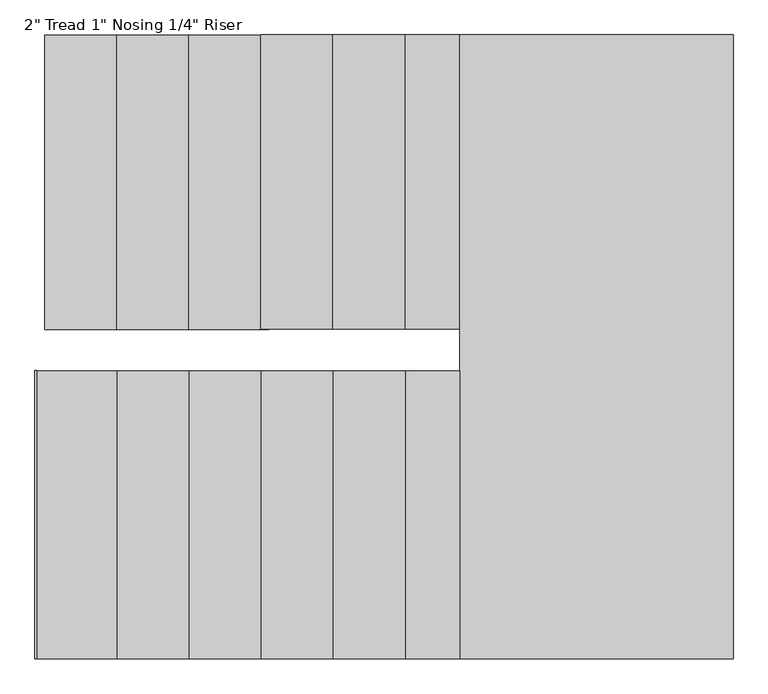
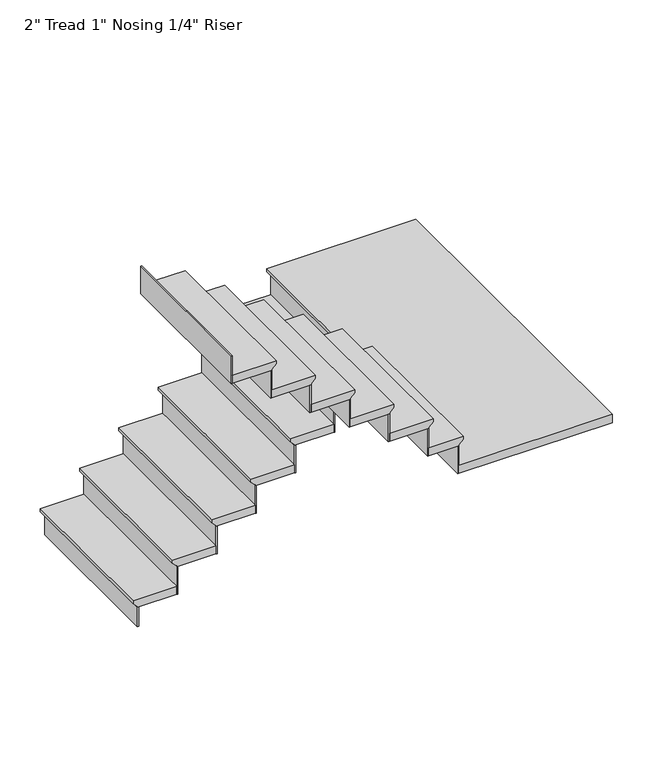
"""IFC4 building model written with IfcOpenShell, lengths in millimetres: stair flight geometry."""

from ifc_helpers import new_model, si_unit, origin, place, context, project, spatial, faceted_brep, source, transform, mapped, element, save


def stair_flight_3a0fea93(model_context):
    return source(origin(), model_context, "Body", "Brep", [
        faceted_brep([(-1022.6415352, -3861.2539367, 150.2833333), (-1022.6415352, -3861.2539367, 169.3333333), (-1022.6415352, -2926.4769687, 169.3333333), (-1022.6415352, -2926.4769687, 150.2833333), (-997.2415352, -3861.2539367, 124.8833333), (-997.2415352, -2926.4769687, 124.8833333), (-768.6415352, -3861.2539367, 169.3333333), (-768.6415352, -2926.4769687, 169.3333333), (-997.2415352, -2926.4769687, 118.5333333), (-768.6415352, -2926.4769687, 118.5333333), (-768.6415352, -3861.2539367, 118.5333333), (-997.2415352, -3861.2539367, 118.5333333)], [[[0, 1, 2, 3]], [[4, 0, 3, 5]], [[2, 1, 6, 7]], [[8, 9, 10, 11]], [[2, 7, 9, 8, 5, 3]], [[8, 11, 4, 5]], [[6, 1, 0, 4, 11, 10]], [[7, 6, 10, 9]]]),
        faceted_brep([(-997.2415352, -3861.2539367, 118.5333333), (-997.2415352, -3861.2539367, 0.0), (-990.8915352, -3861.2539367, 0.0), (-990.8915352, -3861.2539367, 118.5333333), (-997.2415352, -2926.4769687, 118.5333333), (-990.8915352, -2926.4769687, 118.5333333), (-990.8915352, -2926.4769687, 0.0), (-997.2415352, -2926.4769687, 0.0)], [[[0, 1, 2, 3]], [[4, 5, 6, 7]], [[1, 0, 4, 7]], [[2, 1, 7, 6]], [[3, 2, 6, 5]], [[0, 3, 5, 4]]]),
        faceted_brep([(-768.6415352, -3861.2539367, 287.8666667), (-768.6415352, -3861.2539367, 118.5333333), (-762.2915352, -3861.2539367, 118.5333333), (-762.2915352, -3861.2539367, 287.8666667), (-768.6415352, -2926.4769687, 287.8666667), (-762.2915352, -2926.4769687, 287.8666667), (-762.2915352, -2926.4769687, 118.5333333), (-768.6415352, -2926.4769687, 118.5333333)], [[[0, 1, 2, 3]], [[4, 5, 6, 7]], [[1, 0, 4, 7]], [[2, 1, 7, 6]], [[3, 2, 6, 5]], [[0, 3, 5, 4]]]),
        faceted_brep([(-794.0415352, -2926.4769687, 338.6666667), (-794.0415352, -3861.2539367, 338.6666667), (-540.0415352, -3861.2539367, 338.6666667), (-540.0415352, -2926.4769687, 338.6666667), (-768.6415352, -2926.4769687, 287.8666667), (-540.0415352, -2926.4769687, 287.8666667), (-540.0415352, -3861.2539367, 287.8666667), (-768.6415352, -3861.2539367, 287.8666667), (-768.6415352, -2926.4769687, 294.2166667), (-794.0415352, -2926.4769687, 319.6166667), (-768.6415352, -3861.2539367, 294.2166667), (-794.0415352, -3861.2539367, 319.6166667)], [[[0, 1, 2, 3]], [[4, 5, 6, 7]], [[0, 3, 5, 4, 8, 9]], [[4, 7, 10, 8]], [[2, 1, 11, 10, 7, 6]], [[3, 2, 6, 5]], [[11, 1, 0, 9]], [[10, 11, 9, 8]]]),
        faceted_brep([(-540.0415352, -3861.2539367, 457.2), (-540.0415352, -3861.2539367, 287.8666667), (-533.6915352, -3861.2539367, 287.8666667), (-533.6915352, -3861.2539367, 457.2), (-540.0415352, -2926.4769687, 457.2), (-533.6915352, -2926.4769687, 457.2), (-533.6915352, -2926.4769687, 287.8666667), (-540.0415352, -2926.4769687, 287.8666667)], [[[0, 1, 2, 3]], [[4, 5, 6, 7]], [[1, 0, 4, 7]], [[2, 1, 7, 6]], [[3, 2, 6, 5]], [[0, 3, 5, 4]]]),
        faceted_brep([(-565.4415352, -2926.4769687, 508.0), (-565.4415352, -3861.2539367, 508.0), (-311.4415352, -3861.2539367, 508.0), (-311.4415352, -2926.4769687, 508.0), (-540.0415352, -2926.4769687, 457.2), (-311.4415352, -2926.4769687, 457.2), (-311.4415352, -3861.2539367, 457.2), (-540.0415352, -3861.2539367, 457.2), (-540.0415352, -2926.4769687, 463.55), (-565.4415352, -2926.4769687, 488.95), (-540.0415352, -3861.2539367, 463.55), (-565.4415352, -3861.2539367, 488.95)], [[[0, 1, 2, 3]], [[4, 5, 6, 7]], [[0, 3, 5, 4, 8, 9]], [[4, 7, 10, 8]], [[2, 1, 11, 10, 7, 6]], [[3, 2, 6, 5]], [[11, 1, 0, 9]], [[10, 11, 9, 8]]]),
        faceted_brep([(-311.4415352, -3861.2539367, 626.5333333), (-311.4415352, -3861.2539367, 457.2), (-305.0915352, -3861.2539367, 457.2), (-305.0915352, -3861.2539367, 626.5333333), (-311.4415352, -2926.4769687, 626.5333333), (-305.0915352, -2926.4769687, 626.5333333), (-305.0915352, -2926.4769687, 457.2), (-311.4415352, -2926.4769687, 457.2)], [[[0, 1, 2, 3]], [[4, 5, 6, 7]], [[1, 0, 4, 7]], [[2, 1, 7, 6]], [[3, 2, 6, 5]], [[0, 3, 5, 4]]]),
        faceted_brep([(-336.8415352, -2926.4769687, 677.3333333), (-336.8415352, -3861.2539367, 677.3333333), (-82.8415352, -3861.2539367, 677.3333333), (-82.8415352, -2926.4769687, 677.3333333), (-311.4415352, -2926.4769687, 626.5333333), (-82.8415352, -2926.4769687, 626.5333333), (-82.8415352, -3861.2539367, 626.5333333), (-311.4415352, -3861.2539367, 626.5333333), (-311.4415352, -2926.4769687, 632.8833333), (-336.8415352, -2926.4769687, 658.2833333), (-311.4415352, -3861.2539367, 632.8833333), (-336.8415352, -3861.2539367, 658.2833333)], [[[0, 1, 2, 3]], [[4, 5, 6, 7]], [[0, 3, 5, 4, 8, 9]], [[4, 7, 10, 8]], [[2, 1, 11, 10, 7, 6]], [[3, 2, 6, 5]], [[11, 1, 0, 9]], [[10, 11, 9, 8]]]),
        faceted_brep([(-82.8415352, -3861.2539367, 795.8666667), (-82.8415352, -3861.2539367, 626.5333333), (-76.4915352, -3861.2539367, 626.5333333), (-76.4915352, -3861.2539367, 795.8666667), (-82.8415352, -2926.4769687, 795.8666667), (-76.4915352, -2926.4769687, 795.8666667), (-76.4915352, -2926.4769687, 626.5333333), (-82.8415352, -2926.4769687, 626.5333333)], [[[0, 1, 2, 3]], [[4, 5, 6, 7]], [[1, 0, 4, 7]], [[2, 1, 7, 6]], [[3, 2, 6, 5]], [[0, 3, 5, 4]]]),
        faceted_brep([(-108.2415352, -2926.4769687, 846.6666667), (-108.2415352, -3861.2539367, 846.6666667), (145.7584648, -3861.2539367, 846.6666667), (145.7584648, -2926.4769687, 846.6666667), (-82.8415352, -2926.4769687, 795.8666667), (145.7584648, -2926.4769687, 795.8666667), (145.7584648, -3861.2539367, 795.8666667), (-82.8415352, -3861.2539367, 795.8666667), (-82.8415352, -2926.4769687, 802.2166667), (-108.2415352, -2926.4769687, 827.6166667), (-82.8415352, -3861.2539367, 802.2166667), (-108.2415352, -3861.2539367, 827.6166667)], [[[0, 1, 2, 3]], [[4, 5, 6, 7]], [[0, 3, 5, 4, 8, 9]], [[4, 7, 10, 8]], [[2, 1, 11, 10, 7, 6]], [[3, 2, 6, 5]], [[11, 1, 0, 9]], [[10, 11, 9, 8]]]),
        faceted_brep([(145.7584648, -3861.2539367, 965.2), (145.7584648, -3861.2539367, 795.8666667), (152.1084648, -3861.2539367, 795.8666667), (152.1084648, -3861.2539367, 965.2), (145.7584648, -2926.4769687, 965.2), (152.1084648, -2926.4769687, 965.2), (152.1084648, -2926.4769687, 795.8666667), (145.7584648, -2926.4769687, 795.8666667)], [[[0, 1, 2, 3]], [[4, 5, 6, 7]], [[1, 0, 4, 7]], [[2, 1, 7, 6]], [[3, 2, 6, 5]], [[0, 3, 5, 4]]]),
        faceted_brep([(120.3584648, -2926.4769687, 1016.0), (120.3584648, -3861.2539367, 1016.0), (320.0221038, -3861.2539367, 1016.0), (320.0221038, -2926.4769687, 1016.0), (145.7584648, -2926.4769687, 965.2), (320.0221038, -2926.4769687, 965.2), (320.0221038, -3861.2539367, 965.2), (145.7584648, -3861.2539367, 965.2), (145.7584648, -2926.4769687, 971.55), (120.3584648, -2926.4769687, 996.95), (145.7584648, -3861.2539367, 971.55), (120.3584648, -3861.2539367, 996.95)], [[[0, 1, 2, 3]], [[4, 5, 6, 7]], [[0, 3, 5, 4, 8, 9]], [[4, 7, 10, 8]], [[2, 1, 11, 10, 7, 6]], [[3, 2, 6, 5]], [[11, 1, 0, 9]], [[10, 11, 9, 8]]]),
        faceted_brep([(320.0221038, -3861.2539367, 1134.5333333), (320.0221038, -3861.2539367, 965.2), (326.3721038, -3861.2539367, 965.2), (326.3721038, -3861.2539367, 1134.5333333), (320.0221038, -2926.4769687, 1134.5333333), (326.3721038, -2926.4769687, 1134.5333333), (326.3721038, -2926.4769687, 965.2), (320.0221038, -2926.4769687, 965.2)], [[[0, 1, 2, 3]], [[4, 5, 6, 7]], [[1, 0, 4, 7]], [[2, 1, 7, 6]], [[3, 2, 6, 5]], [[0, 3, 5, 4]]]),
        faceted_brep([(269.2221038, -4907.6769687, 1185.3333333), (1161.7584648, -4907.6769687, 1185.3333333), (1161.7584648, -2926.4769687, 1185.3333333), (294.6221038, -2926.4769687, 1185.3333333), (294.6221038, -3993.2769687, 1185.3333333), (269.2221038, -3993.2769687, 1185.3333333), (1161.7584648, -4907.6769687, 1134.5333333), (269.2221038, -4907.6769687, 1134.5333333), (269.2221038, -3993.2769687, 1134.5333333), (294.6221038, -3993.2769687, 1134.5333333), (294.6221038, -3861.2539367, 1134.5333333), (320.0221038, -3861.2539367, 1134.5333333), (320.0221038, -2926.4769687, 1134.5333333), (1161.7584648, -2926.4769687, 1134.5333333), (320.0221038, -2926.4769687, 1140.8833333), (294.6221038, -2926.4769687, 1166.2833333), (320.0221038, -3861.2539367, 1140.8833333), (294.6221038, -3861.2539367, 1166.2833333)], [[[0, 1, 2, 3, 4, 5]], [[6, 7, 8, 9, 10, 11, 12, 13]], [[1, 0, 7, 6]], [[2, 1, 6, 13]], [[3, 2, 13, 12, 14, 15]], [[12, 11, 16, 14]], [[11, 10, 17, 16]], [[4, 3, 15, 17, 10, 9]], [[5, 4, 9, 8]], [[0, 5, 8, 7]], [[15, 14, 16, 17]]]),
        faceted_brep([(269.2221038, -3993.2769687, 1303.8666667), (269.2221038, -3993.2769687, 1134.5333333), (262.8721038, -3993.2769687, 1134.5333333), (262.8721038, -3993.2769687, 1303.8666667), (269.2221038, -4907.6769687, 1303.8666667), (262.8721038, -4907.6769687, 1303.8666667), (262.8721038, -4907.6769687, 1134.5333333), (269.2221038, -4907.6769687, 1134.5333333)], [[[0, 1, 2, 3]], [[4, 5, 6, 7]], [[1, 0, 4, 7]], [[2, 1, 7, 6]], [[3, 2, 6, 5]], [[0, 3, 5, 4]]]),
        faceted_brep([(294.6221038, -4907.6769687, 1354.6666667), (294.6221038, -3993.2769687, 1354.6666667), (94.9584648, -3993.2769687, 1354.6666667), (94.9584648, -4907.6769687, 1354.6666667), (269.2221038, -4907.6769687, 1303.8666667), (94.9584648, -4907.6769687, 1303.8666667), (94.9584648, -3993.2769687, 1303.8666667), (269.2221038, -3993.2769687, 1303.8666667), (269.2221038, -4907.6769687, 1310.2166667), (294.6221038, -4907.6769687, 1335.6166667), (269.2221038, -3993.2769687, 1310.2166667), (294.6221038, -3993.2769687, 1335.6166667)], [[[0, 1, 2, 3]], [[4, 5, 6, 7]], [[0, 3, 5, 4, 8, 9]], [[4, 7, 10, 8]], [[2, 1, 11, 10, 7, 6]], [[3, 2, 6, 5]], [[11, 1, 0, 9]], [[10, 11, 9, 8]]]),
        faceted_brep([(94.9584648, -3993.2769687, 1473.2), (94.9584648, -3993.2769687, 1303.8666667), (88.6084648, -3993.2769687, 1303.8666667), (88.6084648, -3993.2769687, 1473.2), (94.9584648, -4907.6769687, 1473.2), (88.6084648, -4907.6769687, 1473.2), (88.6084648, -4907.6769687, 1303.8666667), (94.9584648, -4907.6769687, 1303.8666667)], [[[0, 1, 2, 3]], [[4, 5, 6, 7]], [[1, 0, 4, 7]], [[2, 1, 7, 6]], [[3, 2, 6, 5]], [[0, 3, 5, 4]]]),
        faceted_brep([(120.3584648, -4907.6769687, 1524.0), (120.3584648, -3993.2769687, 1524.0), (-133.6415352, -3993.2769687, 1524.0), (-133.6415352, -4907.6769687, 1524.0), (94.9584648, -4907.6769687, 1473.2), (-133.6415352, -4907.6769687, 1473.2), (-133.6415352, -3993.2769687, 1473.2), (94.9584648, -3993.2769687, 1473.2), (94.9584648, -4907.6769687, 1479.55), (120.3584648, -4907.6769687, 1504.95), (94.9584648, -3993.2769687, 1479.55), (120.3584648, -3993.2769687, 1504.95)], [[[0, 1, 2, 3]], [[4, 5, 6, 7]], [[0, 3, 5, 4, 8, 9]], [[4, 7, 10, 8]], [[2, 1, 11, 10, 7, 6]], [[3, 2, 6, 5]], [[11, 1, 0, 9]], [[10, 11, 9, 8]]]),
        faceted_brep([(-133.6415352, -3993.2769687, 1642.5333333), (-133.6415352, -3993.2769687, 1473.2), (-139.9915352, -3993.2769687, 1473.2), (-139.9915352, -3993.2769687, 1642.5333333), (-133.6415352, -4907.6769687, 1642.5333333), (-139.9915352, -4907.6769687, 1642.5333333), (-139.9915352, -4907.6769687, 1473.2), (-133.6415352, -4907.6769687, 1473.2)], [[[0, 1, 2, 3]], [[4, 5, 6, 7]], [[1, 0, 4, 7]], [[2, 1, 7, 6]], [[3, 2, 6, 5]], [[0, 3, 5, 4]]]),
        faceted_brep([(-108.2415352, -4907.6769687, 1693.3333333), (-108.2415352, -3993.2769687, 1693.3333333), (-362.2415352, -3993.2769687, 1693.3333333), (-362.2415352, -4907.6769687, 1693.3333333), (-133.6415352, -4907.6769687, 1642.5333333), (-362.2415352, -4907.6769687, 1642.5333333), (-362.2415352, -3993.2769687, 1642.5333333), (-133.6415352, -3993.2769687, 1642.5333333), (-133.6415352, -4907.6769687, 1648.8833333), (-108.2415352, -4907.6769687, 1674.2833333), (-133.6415352, -3993.2769687, 1648.8833333), (-108.2415352, -3993.2769687, 1674.2833333)], [[[0, 1, 2, 3]], [[4, 5, 6, 7]], [[0, 3, 5, 4, 8, 9]], [[4, 7, 10, 8]], [[2, 1, 11, 10, 7, 6]], [[3, 2, 6, 5]], [[11, 1, 0, 9]], [[10, 11, 9, 8]]]),
        faceted_brep([(-362.2415352, -3993.2769687, 1811.8666667), (-362.2415352, -3993.2769687, 1642.5333333), (-368.5915352, -3993.2769687, 1642.5333333), (-368.5915352, -3993.2769687, 1811.8666667), (-362.2415352, -4907.6769687, 1811.8666667), (-368.5915352, -4907.6769687, 1811.8666667), (-368.5915352, -4907.6769687, 1642.5333333), (-362.2415352, -4907.6769687, 1642.5333333)], [[[0, 1, 2, 3]], [[4, 5, 6, 7]], [[1, 0, 4, 7]], [[2, 1, 7, 6]], [[3, 2, 6, 5]], [[0, 3, 5, 4]]]),
        faceted_brep([(-336.8415352, -4907.6769687, 1862.6666667), (-336.8415352, -3993.2769687, 1862.6666667), (-590.8415352, -3993.2769687, 1862.6666667), (-590.8415352, -4907.6769687, 1862.6666667), (-362.2415352, -4907.6769687, 1811.8666667), (-590.8415352, -4907.6769687, 1811.8666667), (-590.8415352, -3993.2769687, 1811.8666667), (-362.2415352, -3993.2769687, 1811.8666667), (-362.2415352, -4907.6769687, 1818.2166667), (-336.8415352, -4907.6769687, 1843.6166667), (-362.2415352, -3993.2769687, 1818.2166667), (-336.8415352, -3993.2769687, 1843.6166667)], [[[0, 1, 2, 3]], [[4, 5, 6, 7]], [[0, 3, 5, 4, 8, 9]], [[4, 7, 10, 8]], [[2, 1, 11, 10, 7, 6]], [[3, 2, 6, 5]], [[11, 1, 0, 9]], [[10, 11, 9, 8]]]),
        faceted_brep([(-590.8415352, -3993.2769687, 1981.2), (-590.8415352, -3993.2769687, 1811.8666667), (-597.1915352, -3993.2769687, 1811.8666667), (-597.1915352, -3993.2769687, 1981.2), (-590.8415352, -4907.6769687, 1981.2), (-597.1915352, -4907.6769687, 1981.2), (-597.1915352, -4907.6769687, 1811.8666667), (-590.8415352, -4907.6769687, 1811.8666667)], [[[0, 1, 2, 3]], [[4, 5, 6, 7]], [[1, 0, 4, 7]], [[2, 1, 7, 6]], [[3, 2, 6, 5]], [[0, 3, 5, 4]]]),
        faceted_brep([(-565.4415352, -4907.6769687, 2032.0), (-565.4415352, -3993.2769687, 2032.0), (-819.4415352, -3993.2769687, 2032.0), (-819.4415352, -4907.6769687, 2032.0), (-590.8415352, -4907.6769687, 1981.2), (-819.4415352, -4907.6769687, 1981.2), (-819.4415352, -3993.2769687, 1981.2), (-590.8415352, -3993.2769687, 1981.2), (-590.8415352, -4907.6769687, 1987.55), (-565.4415352, -4907.6769687, 2012.95), (-590.8415352, -3993.2769687, 1987.55), (-565.4415352, -3993.2769687, 2012.95)], [[[0, 1, 2, 3]], [[4, 5, 6, 7]], [[0, 3, 5, 4, 8, 9]], [[4, 7, 10, 8]], [[2, 1, 11, 10, 7, 6]], [[3, 2, 6, 5]], [[11, 1, 0, 9]], [[10, 11, 9, 8]]]),
        faceted_brep([(-819.4415352, -3993.2769687, 2150.5333333), (-819.4415352, -3993.2769687, 1981.2), (-825.7915352, -3993.2769687, 1981.2), (-825.7915352, -3993.2769687, 2150.5333333), (-819.4415352, -4907.6769687, 2150.5333333), (-825.7915352, -4907.6769687, 2150.5333333), (-825.7915352, -4907.6769687, 1981.2), (-819.4415352, -4907.6769687, 1981.2)], [[[0, 1, 2, 3]], [[4, 5, 6, 7]], [[1, 0, 4, 7]], [[2, 1, 7, 6]], [[3, 2, 6, 5]], [[0, 3, 5, 4]]]),
        faceted_brep([(-1048.0415352, -3993.2769687, 2319.8666667), (-1048.0415352, -3993.2769687, 2150.5333333), (-1054.3915352, -3993.2769687, 2150.5333333), (-1054.3915352, -3993.2769687, 2319.8666667), (-1048.0415352, -4907.6769687, 2319.8666667), (-1054.3915352, -4907.6769687, 2319.8666667), (-1054.3915352, -4907.6769687, 2150.5333333), (-1048.0415352, -4907.6769687, 2150.5333333)], [[[0, 1, 2, 3]], [[4, 5, 6, 7]], [[1, 0, 4, 7]], [[2, 1, 7, 6]], [[3, 2, 6, 5]], [[0, 3, 5, 4]]]),
        faceted_brep([(-794.0415352, -4907.6769687, 2201.3333333), (-794.0415352, -3993.2769687, 2201.3333333), (-1048.0415352, -3993.2769687, 2201.3333333), (-1048.0415352, -4907.6769687, 2201.3333333), (-819.4415352, -4907.6769687, 2150.5333333), (-1048.0415352, -4907.6769687, 2150.5333333), (-1048.0415352, -3993.2769687, 2150.5333333), (-819.4415352, -3993.2769687, 2150.5333333), (-819.4415352, -4907.6769687, 2156.8833333), (-794.0415352, -4907.6769687, 2182.2833333), (-819.4415352, -3993.2769687, 2156.8833333), (-794.0415352, -3993.2769687, 2182.2833333)], [[[0, 1, 2, 3]], [[4, 5, 6, 7]], [[0, 3, 5, 4, 8, 9]], [[4, 7, 10, 8]], [[2, 1, 11, 10, 7, 6]], [[3, 2, 6, 5]], [[11, 1, 0, 9]], [[10, 11, 9, 8]]]),
    ])


if __name__ == "__main__":
    model = new_model("IFC4")
    model_context = context("Model", 3, world=origin())
    ifc_project = project(units=[si_unit("LENGTHUNIT", "METRE", prefix="MILLI")], contexts=[model_context])
    site = spatial("IfcSite", under=ifc_project)
    building = spatial("IfcBuilding", under=site)
    placement = place(None, origin())
    stair_flight_shape = stair_flight_3a0fea93(model_context)
    element("IfcStairFlight", 1, ObjectType="2\" Tread 1\" Nosing 1/4\" Riser", at=placement, inside=building, context=model_context, shape_type="MappedRepresentation", body=[
        mapped(stair_flight_shape, transform((0.0, 0.0, 0.0), x_axis=(1.0, 0.0, 0.0), y_axis=(0.0, 1.0, 0.0), z_axis=(0.0, 0.0, 1.0))),
    ])
    save(model, "model.ifc")
